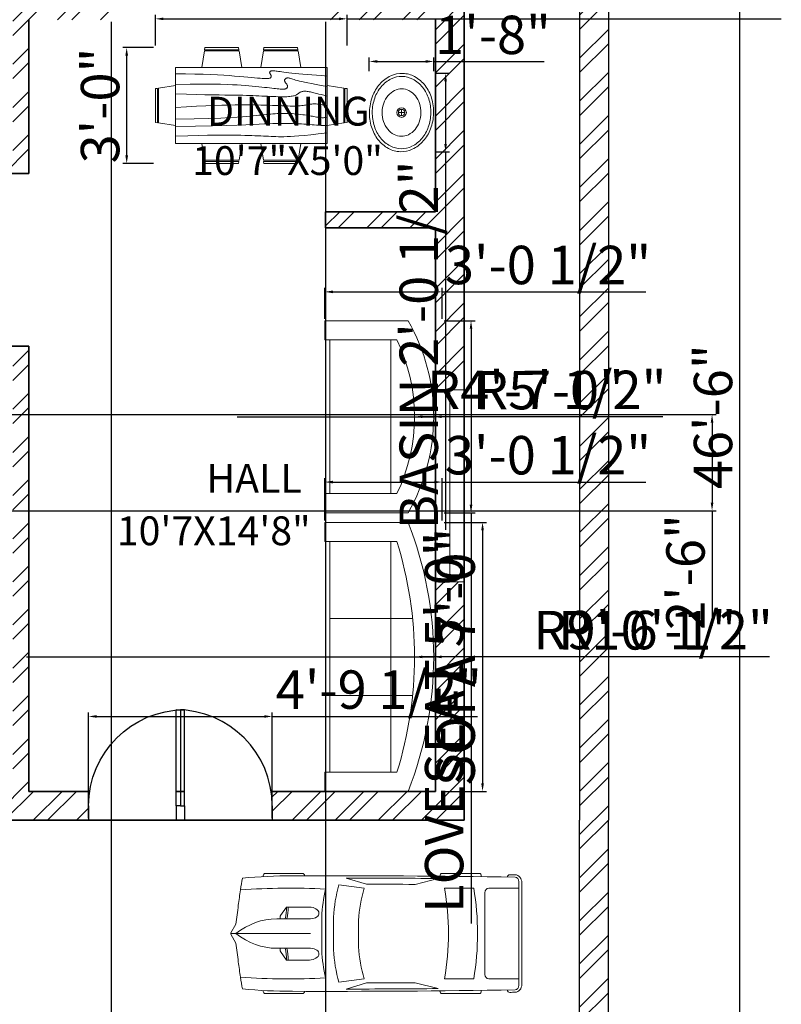
# Model space of a CAD drawing. Units: inches. Extents: x 2588 to 3237, y 2402 to 3178.
# Tile 3 of 4: x 2878 to 3115, y 2568 to 2876. Entities that reach past the tile are written whole.
import ezdxf

# ---------------------------------------------------------------- set-up
doc = ezdxf.new("R2010")
doc.units = ezdxf.units.IN
for name, color, linetype, lineweight in [('A-ANNO-DIMS', 2, 'Continuous', 18), ('A-AREA-IDEN', 7, 'Continuous', 25), ('A-DOOR', 3, 'Continuous', 25), ('A-FLOR-FIXT', 9, 'Continuous', 18), ('A-FURN', 8, 'Continuous', 18), ('A-GLAZ', 4, 'Continuous', 18), ('A-WALL-PATT', 252, 'Continuous', 13), ('C-PRKG-VEHI', 8, 'Continuous', 18), ('L-WALL', 7, 'Continuous', 30), ('L-WALL-PATT', 252, 'Continuous', 13), ('wall', 210, 'Continuous', 35)]:
    doc.layers.add(name, color=color, linetype=linetype, lineweight=lineweight)
doc.styles.get("Standard").update_dxf_attribs({"font": 'arial.ttf'})
doc.dimstyles.new('ISO-25', dxfattribs={"dimtxt": 12, "dimasz": 2.5, "dimexe": 1.25, "dimexo": 0.625, "dimtad": 1, "dimdec": 1, "dimlunit": 4, "dimtxsty": 'Standard', "dimcen": 2.5, "dimadec": 0, "dimazin": 0, "dimtfac": 1, "dimtdec": 1, "dimtmove": 0, "dimatfit": 3, "dimfxl": 1, "dimarcsym": 0})

# ---------------------------------------------------------------- blocks, each defined once
blk = doc.blocks.new('Dining Set - 36 x 72 in.')
for p, q in [((-22.2343, 26.00059), (-23.4847, 17.99762)), ((-22.2304, 26), (-5.7608, 26)), ((-22, 27.5), (-22.1562, 26.50042)), ((-5.8416, 26.5), (-22.1534, 26.5)), ((-22, 27.5), (-6, 27.5)), ((-5.8437, 26.49966), (-6, 27.5)), ((-4.5152, 17.99762), (-5.7655, 25.99926)), ((5.7657, 26.00059), (4.5153, 17.99762)), ((5.7696, 26), (22.2392, 26)), ((6, 27.5), (5.8438, 26.50042)), ((22.1584, 26.5), (5.8466, 26.5)), ((6, 27.5), (22, 27.5)), ((22.1563, 26.49966), (22, 27.5)), ((23.4848, 17.99762), (22.2345, 25.99926)), ((36, 18), (-36, 18)), ((-36, 18), (-36, -18)), ((36, -18), (36, 18)), ((-44.0006, 8.23428), (-35.9976, 9.48474)), ((44.0006, 8.23428), (35.9976, 9.48474)), ((-45.5, 8), (-44.5004, 8.15617)), ((-45.5, 8), (-45.5, -8)), ((-44.5, -8.15843), (-44.5, 8.15338)), ((-44, 8.23041), (-44, -8.23915)), ((44, 8.23041), (44, -8.23915)), ((44.5, -8.15843), (44.5, 8.15338)), ((45.5, 8), (44.5005, 8.15617)), ((45.5, 8), (45.5, -8)), ((-44.4997, -8.15631), (-45.5, -8)), ((-35.9976, -9.48476), (-43.9993, -8.2345)), ((35.9976, -9.48476), (43.9993, -8.2345)), ((44.4997, -8.15631), (45.5, -8)), ((-36, -18), (36, -18)), ((-22.2343, -26.0006), (-23.4847, -17.99762)), ((-4.5152, -17.99762), (-5.7655, -25.99928)), ((5.7657, -26.0006), (4.5153, -17.99762)), ((23.4848, -17.99762), (22.2345, -25.99928)), ((-22.2304, -26), (-5.7608, -26)), ((-22, -27.5), (-22.1562, -26.50044)), ((-5.8416, -26.5), (-22.1534, -26.5)), ((-22, -27.5), (-6, -27.5)), ((-5.8437, -26.49967), (-6, -27.5)), ((5.7696, -26), (22.2392, -26)), ((6, -27.5), (5.8438, -26.50044)), ((22.1584, -26.5), (5.8466, -26.5)), ((6, -27.5), (22, -27.5)), ((22.1563, -26.49967), (22, -27.5))]:
    blk.add_line(p, q)
for points in [[(-36, 15), (-31.1772, 14.97754), (-26.8079, 14.91406), (-22.8538, 14.81543), (-19.276, 14.6875), (-16.0362, 14.53613), (-13.0957, 14.36718), (-10.4159, 14.18652), (-7.9583, 14), (-5.6904, 13.81315), (-3.6035, 13.63021), (-1.6954, 13.45508), (0.0365, 13.29166), (1.5945, 13.14388), (2.9811, 13.01562), (4.1988, 12.9108), (5.25, 12.83333), (6.1393, 12.78613), (6.8802, 12.76823), (7.4883, 12.77767), (7.9792, 12.8125), (8.3685, 12.87077), (8.6719, 12.95052), (8.9049, 13.0498), (9.0833, 13.16666), (9.2205, 13.29899), (9.3216, 13.44401), (9.3895, 13.59879), (9.4271, 13.76041), (9.4373, 13.92594), (9.4232, 14.09245), (9.3875, 14.257), (9.3333, 14.41666), (9.2638, 14.56917), (9.1836, 14.71484), (9.0975, 14.85465), (9.0104, 14.98958), (8.9272, 15.1206), (8.8529, 15.2487), (8.7922, 15.37483), (8.75, 15.5), (8.7305, 15.62467), (8.7344, 15.74739), (8.7617, 15.86621), (8.8125, 15.97916), (8.8867, 16.08431), (8.9844, 16.17968), (9.1055, 16.26334), (9.25, 16.33333), (9.4189, 16.38802), (9.6172, 16.42708), (9.8506, 16.45052), (10.125, 16.45833), (10.4463, 16.45052), (10.8203, 16.42708), (11.2529, 16.38802), (11.75, 16.33333), (12.3184, 16.26318), (12.9694, 16.17838), (13.7151, 16.07991), (14.5677, 15.96875), (15.5395, 15.84586), (16.6426, 15.71224), (17.8893, 15.56884), (19.2917, 15.41666), (20.859, 15.25667), (22.5879, 15.08984), (24.4721, 14.91715), (26.5052, 14.73958), (28.6809, 14.5581), (30.9929, 14.3737), (33.4347, 14.18733), (36, 14)], [(-36, 10), (-28.9766, 10.14274), (-23.1725, 10.20442), (-18.4241, 10.19775), (-14.5677, 10.13541), (-11.4399, 10.03011), (-8.877, 9.89453), (-6.7154, 9.74137), (-4.7917, 9.58333), (-2.9698, 9.43082), (-1.2246, 9.28515), (0.4415, 9.14534), (2.026, 9.01041), (3.5266, 8.87939), (4.9408, 8.7513), (6.266, 8.62516), (7.5, 8.5), (8.6411, 8.37549), (9.6914, 8.2539), (10.6538, 8.13818), (11.5312, 8.03125), (12.3267, 7.93603), (13.043, 7.85547), (13.6831, 7.79248), (14.25, 7.75), (14.7471, 7.7303), (15.1797, 7.73307), (15.5537, 7.75732), (15.875, 7.80208), (16.1494, 7.86637), (16.3828, 7.94922), (16.5811, 8.04964), (16.75, 8.16666), (16.8944, 8.29915), (17.0143, 8.44531), (17.1089, 8.60319), (17.1771, 8.77083), (17.218, 8.94629), (17.2305, 9.1276), (17.2137, 9.31282), (17.1667, 9.5), (17.0895, 9.6875), (16.987, 9.875), (16.8649, 10.0625), (16.7292, 10.25), (16.5856, 10.4375), (16.4401, 10.625), (16.2985, 10.8125), (16.1667, 11), (16.05, 11.18733), (15.9518, 11.3737), (15.8752, 11.5581), (15.8229, 11.73958), (15.798, 11.91715), (15.8034, 12.08984), (15.842, 12.25667), (15.9167, 12.41666), (16.0295, 12.56836), (16.1784, 12.70833), (16.3605, 12.83268), (16.5729, 12.9375), (16.8127, 13.01888), (17.0768, 13.07291), (17.3625, 13.0957), (17.6667, 13.08333), (17.9894, 13.03312), (18.3418, 12.94726), (18.7382, 12.82918), (19.1927, 12.68229), (19.7195, 12.51001), (20.3327, 12.31575), (21.0465, 12.10294), (21.875, 11.875), (22.8357, 11.63354), (23.959, 11.37304), (25.2786, 11.08618), (26.8282, 10.76562), (28.6414, 10.40405), (30.752, 9.99414), (33.1936, 9.52856), (36, 9)], [(-36, 5.5), (-30.7157, 5.3348), (-26.069, 5.20963), (-21.9946, 5.11767), (-18.4271, 5.05208), (-15.3009, 5.00602), (-12.5508, 4.97265), (-10.1112, 4.94515), (-7.9167, 4.91666), (-5.909, 4.88167), (-4.0586, 4.83984), (-2.3429, 4.79215), (-0.7396, 4.73958), (0.7739, 4.6831), (2.22, 4.6237), (3.6213, 4.56233), (5, 4.5), (6.373, 4.43782), (7.7344, 4.3776), (9.0723, 4.32129), (10.375, 4.27083), (11.6309, 4.22819), (12.8281, 4.19531), (13.9551, 4.17415), (15, 4.16666), (15.954, 4.17448), (16.819, 4.19791), (17.6001, 4.23698), (18.3021, 4.29166), (18.9299, 4.36198), (19.4883, 4.44791), (19.9823, 4.54948), (20.4167, 4.66666), (20.7969, 4.79899), (21.1302, 4.94401), (21.4245, 5.09879), (21.6875, 5.26041), (21.9271, 5.42594), (22.1511, 5.59245), (22.3672, 5.757), (22.5834, 5.91666), (22.8065, 6.06868), (23.0404, 6.21093), (23.2879, 6.34147), (23.5521, 6.45833), (23.8358, 6.55957), (24.142, 6.64323), (24.4735, 6.70735), (24.8334, 6.75), (25.2235, 6.76969), (25.642, 6.76692), (26.0858, 6.74267), (26.5521, 6.69791), (27.0379, 6.63362), (27.5404, 6.55078), (28.0565, 6.45036), (28.5834, 6.33333), (29.1242, 6.19987), (29.7071, 6.04687), (30.3661, 5.87044), (31.1354, 5.66666), (32.0493, 5.43164), (33.142, 5.16146), (34.4475, 4.85221), (36, 4.5)], [(-36, -1), (-30.7915, -0.6591), (-26.0195, -0.38216), (-21.6519, -0.16284), (-17.6563, 0.00521), (-14.0005, 0.12833), (-10.6523, 0.21289), (-7.5796, 0.26522), (-4.75, 0.29166), (-2.134, 0.29793), (0.2878, 0.28711), (2.5317, 0.26163), (4.6146, 0.22396), (6.5529, 0.17651), (8.3633, 0.12174), (10.0623, 0.06209), (11.6667, 0), (13.1899, -0.06201), (14.6341, -0.1211), (15.9982, -0.17432), (17.2813, -0.21875), (18.4823, -0.25147), (19.6003, -0.26953), (20.6343, -0.27002), (21.5834, -0.25), (22.4481, -0.20768), (23.2357, -0.14584), (23.9549, -0.06836), (24.6146, 0.02083), (25.2235, 0.11784), (25.7904, 0.21875), (26.3241, 0.31966), (26.8334, 0.41666), (27.3265, 0.50618), (27.8099, 0.58593), (28.2894, 0.65397), (28.7709, 0.70833), (29.2601, 0.74707), (29.763, 0.76823), (30.2855, 0.76985), (30.8334, 0.75), (31.4088, 0.70784), (31.9994, 0.64713), (32.589, 0.57275), (33.1615, 0.48958), (33.7008, 0.4025), (34.1908, 0.3164), (34.6153, 0.23616), (34.9584, 0.16666), (35.2099, 0.11165), (35.3848, 0.07031), (35.504, 0.04069), (35.5886, 0.02083), (35.6594, 0.00879), (35.7377, 0.0026), (35.8442, 0.00032), (36, 0)], [(-36, -6.5), (-27.1843, -6.31267), (-20.084, -6.1263), (-14.469, -5.9419), (-10.1094, -5.76042), (-6.7752, -5.58285), (-4.2363, -5.41016), (-2.2629, -5.24333), (-0.625, -5.08334), (0.8708, -4.93099), (2.2715, -4.78646), (3.5872, -4.64974), (4.8281, -4.52084), (6.0046, -4.39974), (7.127, -4.28646), (8.2053, -4.18099), (9.25, -4.08334), (10.2705, -3.99382), (11.2734, -3.91407), (12.2647, -3.84603), (13.25, -3.79167), (14.2354, -3.75293), (15.2266, -3.73177), (16.2295, -3.73015), (17.25, -3.75), (18.2912, -3.79248), (19.3451, -3.85547), (20.4009, -3.93604), (21.4479, -4.03125), (22.4754, -4.13819), (23.4727, -4.25391), (24.4289, -4.37549), (25.3334, -4.5), (26.1785, -4.62492), (26.9694, -4.74935), (27.7145, -4.87281), (28.4219, -4.99479), (29.1, -5.11483), (29.7572, -5.23242), (30.4016, -5.34709), (31.0417, -5.45834), (31.6837, -5.56437), (32.3262, -5.65821), (32.9658, -5.73153), (33.599, -5.77604), (34.2224, -5.78345), (34.8327, -5.74545), (35.4264, -5.65373), (36, -5.5)], [(-36, -10), (-26.4022, -9.81299), (-18.4675, -9.62891), (-11.9839, -9.45069), (-6.7396, -9.28125), (-2.5226, -9.12354), (0.8789, -8.98047), (3.6769, -8.85498), (6.0833, -8.75), (8.2767, -8.66765), (10.3021, -8.60677), (12.1712, -8.56543), (13.8958, -8.54167), (15.4876, -8.53353), (16.9583, -8.53907), (18.3197, -8.55632), (19.5834, -8.58334), (20.7616, -8.61841), (21.8685, -8.66081), (22.9188, -8.71004), (23.9271, -8.76563), (24.9081, -8.82707), (25.8763, -8.89388), (26.8465, -8.96558), (27.8334, -9.04167), (28.8474, -9.12118), (29.8828, -9.20117), (30.93, -9.27824), (31.9792, -9.34896), (33.0205, -9.40991), (34.0443, -9.45768), (35.0407, -9.48885), (36, -9.5)], [(-36, -14.5), (-30.0881, -14.33513), (-25.0332, -14.21224), (-20.7312, -14.12647), (-17.0781, -14.07292), (-13.97, -14.04671), (-11.3027, -14.04297), (-8.9724, -14.05681), (-6.875, -14.08334), (-4.9224, -14.11833), (-3.0905, -14.16016), (-1.3709, -14.20785), (0.2448, -14.26042), (1.7647, -14.3169), (3.1973, -14.3763), (4.5507, -14.43767), (5.8333, -14.5), (7.0554, -14.5621), (8.235, -14.62175), (9.3922, -14.67652), (10.5469, -14.72396), (11.7192, -14.76164), (12.929, -14.78711), (14.1965, -14.79794), (15.5417, -14.79167), (16.9933, -14.76424), (18.6152, -14.70508), (20.4804, -14.60197), (22.6615, -14.44271), (25.2312, -14.21509), (28.2624, -13.9069), (31.8277, -13.50594), (36, -13)]]:
    blk.add_lwpolyline(points)
blk = doc.blocks.new('Sink - Oval top')
for p, q in [((-1, 0), (1, 0)), ((0, 1), (0, -1))]:
    blk.add_line(p, q)
for points in [[(-12.23, 0.39, 0.117634), (-11.46, -3.36, 0.104469), (-8.88, -6.8, 0.090016), (-5.08, -9.07, 0.08192), (-0.32, -10.02, 0.08192), (4.49, -9.38, 0.090016), (8.42, -7.36, 0.104469), (11.22, -4.09, 0.117634), (12.23, -0.39, 0.117634), (11.46, 3.36, 0.104469), (8.88, 6.8, 0.090016), (5.08, 9.07, 0.08192), (0.32, 10.02, 0.08192), (-4.49, 9.38, 0.090016), (-8.42, 7.36, 0.104469), (-11.22, 4.09, 0.117634)], [(-11.29, 0.16, 0.118622), (-10.52, -3.25, 0.104678), (-8.07, -6.36, 0.089562), (-4.54, -8.37, 0.081185), (-0.13, -9.15, 0.081185), (4.3, -8.49, 0.089562), (7.89, -6.58, 0.104678), (10.42, -3.55, 0.118622), (11.29, -0.16, 0.118622), (10.52, 3.25, 0.104678), (8.07, 6.36, 0.089562), (4.54, 8.37, 0.081185), (0.13, 9.15, 0.081185), (-4.3, 8.49, 0.089562), (-7.89, 6.58, 0.104678), (-10.42, 3.55, 0.118622)], [(-7.42, 0.08, 0.118283), (-6.91, -2.17, 0.104607), (-5.29, -4.21, 0.089718), (-2.97, -5.53, 0.081436), (-0.07, -6.04, 0.081436), (2.84, -5.59, 0.089718), (5.2, -4.33, 0.104607), (6.86, -2.32, 0.118283), (7.42, -0.08, 0.118283), (6.91, 2.17, 0.104607), (5.29, 4.21, 0.089718), (2.97, 5.53, 0.081436), (0.07, 6.04, 0.081436), (-2.84, 5.59, 0.089718), (-5.2, 4.33, 0.104607), (-6.86, 2.32, 0.118283)]]:
    blk.add_lwpolyline(points, format="xyb", close=True)
for radius in [1.5, 1]:
    blk.add_circle((0, 0), radius)
blk = doc.blocks.new('*U14')
for p, q in [((0, 0), (0, -6)), ((40, 0), (40, -6))]:
    blk.add_line(p, q)
blk.add_lwpolyline([(0, 0), (0, 40), (1.75, 40), (1.75, 0)], close=True)
blk.add_arc((0, 0), 40, 0, 90)
blk = doc.blocks.new('Sofa - Roundback 7 ft.')
for p, q in [((-12.00002, -32.4421), (-12.00003, -6.5971)), ((11.99997, -32.4421), (11.99998, -6.5971)), ((-36.000027, -34), (-36.000027, -11.4696)), ((35.99998, -34), (35.99998, -11.4696)), ((-35.999844, -13.3819), (35.9998, -13.3819)), ((-36.000027, -32.4421), (35.99998, -32.4421))]:
    blk.add_line(p, q)
for points in [[(-36.000027, -34), (-42.000027, -34), (-42.000027, -8)], [(41.99998, -8), (41.99998, -34), (35.99998, -34)]]:
    blk.add_lwpolyline(points)
for centre, radius, start, end in [((0, -114.25), 114.25, 68.43141, 111.5686), ((-0.00001, -127.1968), 121.1968, 72.72033, 107.2797)]:
    blk.add_arc(centre, radius, start, end)
blk = doc.blocks.new('Sofa - Roundback Loveseat 5 ft.')
for p, q in [((0, -32.44198), (0, -5.99998)), ((-24, -33.99998), (-24, -11.46958)), ((24.00004, -33.99998), (24.00004, -11.46958)), ((-23.9998, -13.38178), (23.99986, -13.38178)), ((-24, -32.44198), (24.00004, -32.44198))]:
    blk.add_line(p, q)
for points in [[(-24, -33.99998), (-30, -33.99998), (-30, -7.99998)], [(30.00004, -7.99998), (30.00004, -33.99998), (24.00004, -33.99998)]]:
    blk.add_lwpolyline(points)
for centre, radius, start, end in [((0, -60.24998), 60.24998, 60.13715, 119.8628), ((0, -61.38438), 55.38444, 64.32083, 115.6792)]:
    blk.add_arc(centre, radius, start, end)
blk = doc.blocks.new('*U21')
for p, q in [((46.55, 38.89), (22.35, 38.89)), ((136.7, 38.89), (160.9, 38.89)), ((21.1, 37.41), (21.1, 36.83)), ((47.8, 37.39), (47.8, 37.41)), ((87.99, 31.87), (74.76, 35.92)), ((134.31, 35.6), (119.29, 31.78)), ((135.45, 37.07), (135.45, 37.41)), ((162.15, 37.41), (162.15, 36.77)), ((186.47, -33.5), (186.47, 33.5)), ((188.4, -32.76), (188.4, 32.76)), ((70.03, 31.54), (86.41, 29.35)), ((138.42, 29.35), (157.25, 29.35)), ((164.52, 26.39), (164.52, -26.39)), ((186.47, 29.35), (167.01, 29.35)), ((32.27, 11.63), (36.13, 17.17)), ((36.13, 17.17), (50.94, 17.17)), ((29.77, 9.51), (51.68, 9.51)), ((32.12, 9.51), (32.12, 11.15)), ((58.92, -10.77), (58.92, 10.77)), ((66.55, -10.53), (66.55, 10.53)), ((82.74, 8.5), (82.74, -8.5)), ((186.47, -10.53), (186.47, 10.53)), ((3.27, 6.13), (0.1, 0.41)), ((0, 0), (51.68, 0)), ((0.1, -0.41), (3.27, -6.13)), ((29.77, -9.51), (51.68, -9.51)), ((32.12, -9.51), (32.12, -11.15)), ((32.27, -11.63), (36.13, -17.17)), ((36.13, -17.17), (50.94, -17.17)), ((86.41, -29.35), (70.03, -31.54)), ((134.31, -35.6), (119.29, -31.78)), ((157.25, -29.35), (138.42, -29.35)), ((167.01, -29.35), (186.47, -29.35)), ((21.1, -37.41), (21.1, -36.83)), ((47.8, -37.39), (47.8, -37.41)), ((87.99, -31.87), (74.76, -35.92)), ((135.45, -37.07), (135.45, -37.41)), ((162.15, -37.41), (162.15, -36.77)), ((46.55, -38.89), (22.35, -38.89)), ((136.7, -38.89), (160.9, -38.89))]:
    blk.add_line(p, q)
for centre, major_axis, ratio, start_param, end_param in [((22.35, 37.41), (0, -1.48), 0.842304, 3.141593, 4.712389), ((46.55, 37.41), (0, 1.48), 0.842304, -1.570796, 0), ((136.7, 37.41), (0, -1.48), 0.842304, 3.141593, 4.712389), ((160.9, 37.41), (0, 1.48), 0.842304, -1.570796, 0), ((266.03, -27.52), (0, 313.31), 0.842304, 1.367076, 1.39176), ((41.19, -490.86), (0, 528.23), 0.842304, 0.00281, 0.075598), ((64.48, -10555.62), (0, 10593.03), 0.842304, -0.013397, 0.002797), ((64.48, -10555.62), (0, -10591.55), 0.842304, 3.133765, 3.140441), ((95.79, -3666.35), (0, -3698.24), 0.842304, 3.134049, 3.144098), ((180.63, 35.84), (0, 2.22), 0.842304, -0.013017, 1.249894), ((64.48, -10556.36), (0, 10595.31), 0.842304, -0.013397, -0.013017), ((183.98, 33.5), (0, -2.96), 0.842304, 1.570796, 3.128196), ((183.98, 32.76), (0, -5.25), 0.842304, 1.570796, 3.128196), ((259.18, -27.52), (0, -305.3), 0.842304, 4.528606, 4.561838), ((37.47, -593.96), (0, -623.33), 0.842304, 3.096046, 3.200911), ((134.4, 5.39), (0, -89.78), 0.842304, 4.449482, 4.652344), ((135.29, 5.39), (0, 81.77), 0.842304, 1.245306, 1.50788), ((149.6, 2.8), (0, -79.58), 0.842304, 4.372215, 4.640744), ((17.08, 0), (0, 147.02), 0.842304, 4.511394, 4.913384), ((35.91, 0), (0, 147.02), 0.842304, 4.511394, 4.913384), ((167.01, 26.39), (0, 2.96), 0.842304, 0, 1.570796), ((-204.49, 52.4), (0, -250.96), 0.842304, 1.385369, 1.434372), ((13.04, 17.01), (0, 27.42), 0.842304, 4.435146, 4.718221), ((14.2, 17.01), (0, 27.42), 0.842304, 4.435146, 4.718221), ((50.79, 13.34), (6.34, -0.36), 0.603834, -1.395552, 1.581315), ((29.77, -46.66), (0, 56.17), 0.842304, 0, 0.590319), ((32.75, 11.15), (0, 0.74), 0.842304, 0.879714, 1.570796), ((0.62, 0), (0, -0.74), 0.842304, 4.131459, 5.293319), ((-204.49, -52.4), (0, 250.96), 0.842304, -1.434372, -1.385369), ((29.77, 46.66), (0, 56.17), 0.842304, 2.551274, 3.141593), ((32.75, -11.15), (0, -0.74), 0.842304, 4.712389, 5.403472), ((13.04, -17.01), (0, -27.42), 0.842304, 1.564964, 1.848039), ((14.2, -17.01), (0, -27.42), 0.842304, 1.564964, 1.848039), ((134.4, -5.39), (0, -89.78), 0.842304, -1.510751, -1.307889), ((135.29, -5.39), (0, -81.77), 0.842304, -1.50788, -1.245306), ((149.6, -2.8), (0, -79.58), 0.842304, -1.499151, -1.230623), ((259.18, 27.52), (0, 305.3), 0.842304, 1.721348, 1.754579), ((266.03, 27.52), (0, 313.31), 0.842304, 1.749832, 1.774517), ((37.47, 593.96), (0, -623.33), 0.842304, -0.059319, 0.045547), ((95.79, 3666.35), (0, -3698.24), 0.842304, -0.002505, 0.007544), ((167.01, -26.39), (0, -2.96), 0.842304, 4.712389, 6.283185), ((41.19, 490.86), (0, -528.23), 0.842304, -0.075598, -0.00281), ((22.35, -37.41), (0, 1.48), 0.842304, 1.570796, 3.141593), ((64.48, 10555.62), (0, 10593.03), 0.842304, 3.138796, 3.15499), ((46.55, -37.41), (0, -1.48), 0.842304, 0, 1.570796), ((64.48, 10555.62), (0, -10591.55), 0.842304, 0.001152, 0.007828), ((136.7, -37.41), (0, -1.48), 0.842304, -1.570796, 0), ((160.9, -37.41), (0, 1.48), 0.842304, 3.141593, 4.712389), ((180.63, -35.84), (0, -2.22), 0.842304, -1.249894, 0.013017), ((64.48, 10556.36), (0, 10595.31), 0.842304, 3.15461, 3.15499), ((183.98, -33.5), (0, 2.96), 0.842304, 3.15499, 4.712389), ((183.98, -32.76), (0, -5.25), 0.842304, 0.013397, 1.570796)]:
    blk.add_ellipse(centre, major_axis=major_axis, ratio=ratio, start_param=start_param, end_param=end_param)
at = {"extrusion": (0, 0, -1)}
blk.add_ellipse((50.79, -13.34), major_axis=(6.34, 0.36), ratio=0.603834, start_param=-1.395552, end_param=1.581315, dxfattribs=at)
blk = doc.blocks.new('*D23')
at = {"layer": 'A-ANNO-DIMS', "color": 0, "lineweight": -2, "transparency": 16777216}
for p, q in [((3062.02, 3030.83), (3103.65, 3030.83)), ((3102.4, 3028.33), (3102.4, 2475.33)), ((3062.02, 2472.83), (3103.65, 2472.83))]:
    blk.add_line(p, q, dxfattribs=at)
at = {"layer": 'A-ANNO-DIMS', "color": 0, "transparency": 16777216}
for points in [[(3101.99, 3028.33), (3102.82, 3028.33), (3102.4, 3030.83)], [(3101.99, 2475.33), (3102.82, 2475.33), (3102.4, 2472.83)]]:
    blk.add_solid(points, dxfattribs=at)
at = {"layer": 'Defpoints', "color": 0, "transparency": 16777216}
for p in [(3061.4, 3030.83), (3061.4, 2472.83), (3102.4, 2472.83)]:
    blk.add_point(p, dxfattribs=at)
at = {"layer": 'A-ANNO-DIMS', "color": 0, "transparency": 16777216, "insert": (3095.65, 2751.83), "char_height": 12, "attachment_point": 5, "rotation": 90}
blk.add_mtext('46\'-6"', dxfattribs=at)
blk = doc.blocks.new('WIN-60IN')
blk.add_line((4.5, 60), (4.5, 0))
blk.add_lwpolyline([(9, 60), (9, 0), (0, 0), (0, 60)], close=True)
blk = doc.blocks.new('*D29')
at = {"layer": 'A-ANNO-DIMS', "color": 0, "lineweight": -2, "transparency": 16777216}
for p, q in [((2761.13, 2894.89), (2761.13, 2882.27)), ((2821.13, 2894.89), (2821.13, 2882.27)), ((2763.63, 2883.52), (2818.63, 2883.52)), ((2821.13, 2883.52), (2898.03, 2883.52))]:
    blk.add_line(p, q, dxfattribs=at)
at = {"layer": 'A-ANNO-DIMS', "color": 0, "transparency": 16777216}
for points in [[(2763.63, 2883.93), (2763.63, 2883.1), (2761.13, 2883.52)], [(2818.63, 2883.93), (2818.63, 2883.1), (2821.13, 2883.52)]]:
    blk.add_solid(points, dxfattribs=at)
at = {"layer": 'Defpoints', "color": 0, "transparency": 16777216}
for p in [(2761.13, 2895.52), (2821.13, 2895.52), (2821.13, 2883.52)]:
    blk.add_point(p, dxfattribs=at)
at = {"layer": 'A-ANNO-DIMS', "color": 0, "transparency": 16777216, "insert": (2860.83, 2890.27), "char_height": 12, "attachment_point": 5}
blk.add_mtext('5\'-0" TYP.', dxfattribs=at)
blk = doc.blocks.new('*D36')
at = {"layer": 'A-ANNO-DIMS', "color": 0, "lineweight": -2, "transparency": 16777216}
for p, q in [((2919.92, 2867.74), (2919.92, 2877.35)), ((2922.42, 2876.1), (2977.29, 2876.1)), ((2979.79, 2867.74), (2979.79, 2877.35)), ((2979.79, 2876.1), (3115.43, 2876.1))]:
    blk.add_line(p, q, dxfattribs=at)
at = {"layer": 'A-ANNO-DIMS', "color": 0, "transparency": 16777216}
for points in [[(2922.42, 2876.51), (2922.42, 2875.68), (2919.92, 2876.1)], [(2977.29, 2876.51), (2977.29, 2875.68), (2979.79, 2876.1)]]:
    blk.add_solid(points, dxfattribs=at)
at = {"layer": 'Defpoints', "color": 0, "transparency": 16777216}
for p in [(2979.79, 2876.1), (2919.92, 2867.12), (2979.79, 2867.12)]:
    blk.add_point(p, dxfattribs=at)
at = {"layer": 'A-ANNO-DIMS', "color": 0, "transparency": 16777216, "insert": (3048.86, 2882.93), "char_height": 12, "attachment_point": 5}
blk.add_mtext('DINING SET 5\'-0"', dxfattribs=at)
blk = doc.blocks.new('*D37')
at = {"layer": 'A-ANNO-DIMS', "color": 0, "lineweight": -2, "transparency": 16777216}
for p, q in [((2919.3, 2867.12), (2909.69, 2867.12)), ((2910.94, 2833.44), (2910.94, 2864.62)), ((2919.3, 2830.94), (2909.69, 2830.94))]:
    blk.add_line(p, q, dxfattribs=at)
at = {"layer": 'A-ANNO-DIMS', "color": 0, "transparency": 16777216}
for points in [[(2910.53, 2864.62), (2911.36, 2864.62), (2910.94, 2867.12)], [(2910.53, 2833.44), (2911.36, 2833.44), (2910.94, 2830.94)]]:
    blk.add_solid(points, dxfattribs=at)
at = {"layer": 'Defpoints', "color": 0, "transparency": 16777216}
for p in [(2910.94, 2867.12), (2919.92, 2867.12), (2919.92, 2830.94)]:
    blk.add_point(p, dxfattribs=at)
at = {"layer": 'A-ANNO-DIMS', "color": 0, "transparency": 16777216, "insert": (2904.19, 2849.03), "char_height": 12, "attachment_point": 5, "rotation": 90}
blk.add_mtext('3\'-0"', dxfattribs=at)
blk = doc.blocks.new('*D38')
at = {"layer": 'A-ANNO-DIMS', "color": 0, "lineweight": -2, "transparency": 16777216}
for p, q in [((3007.49, 2859.11), (3011.8, 2859.11)), ((3010.55, 2856.61), (3010.55, 2837.06)), ((3007.49, 2834.56), (3011.8, 2834.56)), ((3010.55, 2834.56), (3010.55, 2716.51))]:
    blk.add_line(p, q, dxfattribs=at)
at = {"layer": 'A-ANNO-DIMS', "color": 0, "transparency": 16777216}
for points in [[(3010.14, 2856.61), (3010.97, 2856.61), (3010.55, 2859.11)], [(3010.14, 2837.06), (3010.97, 2837.06), (3010.55, 2834.56)]]:
    blk.add_solid(points, dxfattribs=at)
at = {"layer": 'Defpoints', "color": 0, "transparency": 16777216}
for p in [(3006.87, 2859.11), (3006.87, 2834.56), (3010.55, 2834.56)]:
    blk.add_point(p, dxfattribs=at)
at = {"layer": 'A-ANNO-DIMS', "color": 0, "transparency": 16777216, "insert": (3003.72, 2774.28), "char_height": 12, "attachment_point": 5, "rotation": 90}
blk.add_mtext('BASIN 2\'-0 1/2"', dxfattribs=at)
blk = doc.blocks.new('*D39')
at = {"layer": 'A-ANNO-DIMS', "color": 0, "lineweight": -2, "transparency": 16777216}
for p, q in [((2986.73, 2859.73), (2986.73, 2864.04)), ((2989.23, 2862.79), (3004.37, 2862.79)), ((3006.87, 2859.73), (3006.87, 2864.04)), ((3006.87, 2862.79), (3041.39, 2862.79))]:
    blk.add_line(p, q, dxfattribs=at)
at = {"layer": 'A-ANNO-DIMS', "color": 0, "transparency": 16777216}
for points in [[(2989.23, 2863.21), (2989.23, 2862.37), (2986.73, 2862.79)], [(3004.37, 2863.21), (3004.37, 2862.37), (3006.87, 2862.79)]]:
    blk.add_solid(points, dxfattribs=at)
at = {"layer": 'Defpoints', "color": 0, "transparency": 16777216}
for p in [(3006.87, 2862.79), (2986.73, 2859.11), (3006.87, 2859.11)]:
    blk.add_point(p, dxfattribs=at)
at = {"layer": 'A-ANNO-DIMS', "color": 0, "transparency": 16777216, "insert": (3025.38, 2869.54), "char_height": 12, "attachment_point": 5}
blk.add_mtext('1\'-8"', dxfattribs=at)
blk = doc.blocks.new('*D42')
at = {"layer": 'A-ANNO-DIMS', "color": 0, "lineweight": -2, "transparency": 16777216}
for p, q in [((3010.13, 2718.83), (3023.36, 2718.83)), ((3022.11, 2716.33), (3022.11, 2637.33)), ((3010.13, 2634.83), (3023.36, 2634.83))]:
    blk.add_line(p, q, dxfattribs=at)
at = {"layer": 'A-ANNO-DIMS', "color": 0, "transparency": 16777216}
for points in [[(3021.69, 2716.33), (3022.52, 2716.33), (3022.11, 2718.83)], [(3021.69, 2637.33), (3022.52, 2637.33), (3022.11, 2634.83)]]:
    blk.add_solid(points, dxfattribs=at)
at = {"layer": 'Defpoints', "color": 0, "transparency": 16777216}
for p in [(3009.51, 2718.83), (3009.51, 2634.83), (3022.11, 2634.83)]:
    blk.add_point(p, dxfattribs=at)
at = {"layer": 'A-ANNO-DIMS', "color": 0, "transparency": 16777216, "insert": (3015.27, 2676.83), "char_height": 12, "attachment_point": 5, "rotation": 90}
blk.add_mtext('SOFA 7\'-0"', dxfattribs=at)
blk = doc.blocks.new('*D43')
at = {"layer": 'A-ANNO-DIMS', "color": 0, "lineweight": -2, "transparency": 16777216}
for p, q in [((2972.84, 2719.46), (2972.84, 2732.68)), ((2975.34, 2731.43), (3007.01, 2731.43)), ((3009.51, 2719.46), (3009.51, 2732.68)), ((3009.51, 2731.43), (3073.11, 2731.43))]:
    blk.add_line(p, q, dxfattribs=at)
at = {"layer": 'A-ANNO-DIMS', "color": 0, "transparency": 16777216}
for points in [[(2975.34, 2731.85), (2975.34, 2731.02), (2972.84, 2731.43)], [(3007.01, 2731.85), (3007.01, 2731.02), (3009.51, 2731.43)]]:
    blk.add_solid(points, dxfattribs=at)
at = {"layer": 'Defpoints', "color": 0, "transparency": 16777216}
for p in [(3009.51, 2731.43), (2972.84, 2718.83), (3009.51, 2718.83)]:
    blk.add_point(p, dxfattribs=at)
at = {"layer": 'A-ANNO-DIMS', "color": 0, "transparency": 16777216, "insert": (3042.56, 2738.27), "char_height": 12, "attachment_point": 5}
blk.add_mtext('3\'-0 1/2"', dxfattribs=at)
blk = doc.blocks.new('*D44')
at = {"layer": 'A-ANNO-DIMS', "color": 0, "lineweight": -2, "transparency": 16777216}
for p, q in [((3010.13, 2781.83), (3019.76, 2781.83)), ((3018.51, 2779.33), (3018.51, 2724.33)), ((3010.13, 2721.83), (3019.76, 2721.83)), ((3018.51, 2721.83), (3018.51, 2593.55))]:
    blk.add_line(p, q, dxfattribs=at)
at = {"layer": 'A-ANNO-DIMS', "color": 0, "transparency": 16777216}
for points in [[(3018.09, 2779.33), (3018.92, 2779.33), (3018.51, 2781.83)], [(3018.09, 2724.33), (3018.92, 2724.33), (3018.51, 2721.83)]]:
    blk.add_solid(points, dxfattribs=at)
at = {"layer": 'Defpoints', "color": 0, "transparency": 16777216}
for p in [(3009.51, 2781.83), (3009.51, 2721.83), (3018.51, 2721.83)]:
    blk.add_point(p, dxfattribs=at)
at = {"layer": 'A-ANNO-DIMS', "color": 0, "transparency": 16777216, "insert": (3011.67, 2656.44), "char_height": 12, "attachment_point": 5, "rotation": 90}
blk.add_mtext('LOVESEAT 5\'-0"', dxfattribs=at)
blk = doc.blocks.new('*D45')
at = {"layer": 'A-ANNO-DIMS', "color": 0, "lineweight": -2, "transparency": 16777216}
for p, q in [((2972.84, 2782.46), (2972.84, 2792.08)), ((3009.51, 2782.46), (3009.51, 2792.08)), ((2975.34, 2790.83), (3007.01, 2790.83)), ((3009.51, 2790.83), (3073.11, 2790.83))]:
    blk.add_line(p, q, dxfattribs=at)
at = {"layer": 'A-ANNO-DIMS', "color": 0, "transparency": 16777216}
for points in [[(2975.34, 2791.25), (2975.34, 2790.42), (2972.84, 2790.83)], [(3007.01, 2791.25), (3007.01, 2790.42), (3009.51, 2790.83)]]:
    blk.add_solid(points, dxfattribs=at)
at = {"layer": 'Defpoints', "color": 0, "transparency": 16777216}
for p in [(3009.51, 2790.83), (2972.84, 2781.83), (3009.51, 2781.83)]:
    blk.add_point(p, dxfattribs=at)
at = {"layer": 'A-ANNO-DIMS', "color": 0, "transparency": 16777216, "insert": (3042.56, 2797.67), "char_height": 12, "attachment_point": 5}
blk.add_mtext('3\'-0 1/2"', dxfattribs=at)
blk = doc.blocks.new('*D56')
at = {"layer": 'A-ANNO-DIMS', "color": 0, "lineweight": -2, "transparency": 16777216}
for p, q in [((2821.33, 2752.5), (3095.05, 2752.5)), ((3093.8, 2750), (3093.8, 2725)), ((2821.33, 2722.5), (3095.05, 2722.5)), ((3093.8, 2722.5), (3093.8, 2686.65))]:
    blk.add_line(p, q, dxfattribs=at)
at = {"layer": 'A-ANNO-DIMS', "color": 0, "transparency": 16777216}
for points in [[(3093.38, 2750), (3094.21, 2750), (3093.8, 2752.5)], [(3093.38, 2725), (3094.21, 2725), (3093.8, 2722.5)]]:
    blk.add_solid(points, dxfattribs=at)
at = {"layer": 'Defpoints', "color": 0, "transparency": 16777216}
for p in [(2820.7, 2752.5), (2820.7, 2722.5), (3093.8, 2722.5)]:
    blk.add_point(p, dxfattribs=at)
at = {"layer": 'A-ANNO-DIMS', "color": 0, "transparency": 16777216, "insert": (3087.05, 2703.33), "char_height": 12, "attachment_point": 5, "rotation": 90}
blk.add_mtext('2\'-6"', dxfattribs=at)
blk = doc.blocks.new('*D57')
at = {"layer": 'A-ANNO-DIMS', "color": 0, "lineweight": -2, "transparency": 16777216}
for p, q in [((2906.11, 2875.21), (2906.11, 2412.16)), ((2973.06, 2875.21), (2973.06, 2412.16)), ((2908.61, 2413.41), (2970.56, 2413.41))]:
    blk.add_line(p, q, dxfattribs=at)
at = {"layer": 'A-ANNO-DIMS', "color": 0, "transparency": 16777216}
for points in [[(2908.61, 2413.83), (2908.61, 2412.99), (2906.11, 2413.41)], [(2970.56, 2413.83), (2970.56, 2412.99), (2973.06, 2413.41)]]:
    blk.add_solid(points, dxfattribs=at)
at = {"layer": 'Defpoints', "color": 0, "transparency": 16777216}
for p in [(2906.11, 2875.83), (2973.06, 2875.83), (2973.06, 2413.41)]:
    blk.add_point(p, dxfattribs=at)
at = {"layer": 'A-ANNO-DIMS', "color": 0, "transparency": 16777216, "insert": (2939.58, 2420.14), "char_height": 12, "attachment_point": 5}
blk.add_mtext('5\'-7"', dxfattribs=at)
blk = doc.blocks.new('*D59')
at = {"layer": 'A-ANNO-DIMS', "color": 0, "lineweight": -2, "transparency": 16777216}
for p, q in [((2899.05, 2626.46), (2899.05, 2659.48)), ((2901.55, 2658.23), (2953.92, 2658.23)), ((2956.42, 2626.46), (2956.42, 2659.48)), ((2956.42, 2658.23), (3020.52, 2658.23))]:
    blk.add_line(p, q, dxfattribs=at)
at = {"layer": 'A-ANNO-DIMS', "color": 0, "transparency": 16777216}
for points in [[(2901.55, 2658.65), (2901.55, 2657.82), (2899.05, 2658.23)], [(2953.92, 2658.65), (2953.92, 2657.82), (2956.42, 2658.23)]]:
    blk.add_solid(points, dxfattribs=at)
at = {"layer": 'Defpoints', "color": 0, "transparency": 16777216}
for p in [(2956.42, 2658.23), (2899.05, 2625.83), (2956.42, 2625.83)]:
    blk.add_point(p, dxfattribs=at)
at = {"layer": 'A-ANNO-DIMS', "color": 0, "transparency": 16777216, "insert": (2989.72, 2665.06), "char_height": 12, "attachment_point": 5}
blk.add_mtext('4\'-9 1/2"', dxfattribs=at)
blk = doc.blocks.new('*D60')
at = {"layer": 'A-ANNO-DIMS', "color": 0, "lineweight": -2, "transparency": 16777216}
for p, q in [((2879.64, 2676.83), (3000.84, 2676.83)), ((3100.54, 2676.83), (3003.34, 2676.83))]:
    blk.add_line(p, q, dxfattribs=at)
at = {"layer": 'A-ANNO-DIMS', "color": 0, "transparency": 16777216}
blk.add_solid([(3003.34, 2677.25), (3003.34, 2676.42), (3000.84, 2676.83)], dxfattribs=at)
at = {"layer": 'Defpoints', "color": 0, "transparency": 16777216}
for p in [(2879.64, 2676.83), (3000.84, 2676.83)]:
    blk.add_point(p, dxfattribs=at)
at = {"layer": 'A-ANNO-DIMS', "color": 0, "transparency": 16777216, "insert": (3073.56, 2683.58), "char_height": 12, "attachment_point": 5, "rotation": 360}
blk.add_mtext('R10\'-1"', dxfattribs=at)
blk = doc.blocks.new('*D61')
at = {"layer": 'A-ANNO-DIMS', "color": 0, "lineweight": -2, "transparency": 16777216}
for p, q in [((2892.59, 2676.83), (3006.84, 2676.83)), ((3111.69, 2676.83), (3009.34, 2676.83))]:
    blk.add_line(p, q, dxfattribs=at)
at = {"layer": 'A-ANNO-DIMS', "color": 0, "transparency": 16777216}
blk.add_solid([(3009.34, 2677.25), (3009.34, 2676.42), (3006.84, 2676.83)], dxfattribs=at)
at = {"layer": 'Defpoints', "color": 0, "transparency": 16777216}
for p in [(2892.59, 2676.83), (3006.84, 2676.83)]:
    blk.add_point(p, dxfattribs=at)
at = {"layer": 'A-ANNO-DIMS', "color": 0, "transparency": 16777216, "insert": (3075.39, 2683.66), "char_height": 12, "attachment_point": 5, "rotation": 360}
blk.add_mtext('R9\'-6 1/2"', dxfattribs=at)
blk = doc.blocks.new('*D62')
at = {"layer": 'A-ANNO-DIMS', "color": 0, "lineweight": -2, "transparency": 16777216}
for p, q in [((2946.59, 2751.83), (3006.84, 2751.83)), ((3065.31, 2751.83), (3009.34, 2751.83))]:
    blk.add_line(p, q, dxfattribs=at)
at = {"layer": 'A-ANNO-DIMS', "color": 0, "transparency": 16777216}
blk.add_solid([(3009.34, 2752.25), (3009.34, 2751.42), (3006.84, 2751.83)], dxfattribs=at)
at = {"layer": 'Defpoints', "color": 0, "transparency": 16777216}
for p in [(2946.59, 2751.83), (3006.84, 2751.83)]:
    blk.add_point(p, dxfattribs=at)
at = {"layer": 'A-ANNO-DIMS', "color": 0, "transparency": 16777216, "insert": (3042.99, 2758.59), "char_height": 12, "attachment_point": 5, "rotation": 0}
blk.add_mtext('R5\'-0"', dxfattribs=at)
blk = doc.blocks.new('*D63')
at = {"layer": 'A-ANNO-DIMS', "color": 0, "lineweight": -2, "transparency": 16777216}
for p, q in [((2945.46, 2751.83), (3000.84, 2751.83)), ((3078.44, 2751.83), (3003.34, 2751.83))]:
    blk.add_line(p, q, dxfattribs=at)
at = {"layer": 'A-ANNO-DIMS', "color": 0, "transparency": 16777216}
blk.add_solid([(3003.34, 2752.25), (3003.34, 2751.42), (3000.84, 2751.83)], dxfattribs=at)
at = {"layer": 'Defpoints', "color": 0, "transparency": 16777216}
for p in [(2945.46, 2751.83), (3000.84, 2751.83)]:
    blk.add_point(p, dxfattribs=at)
at = {"layer": 'A-ANNO-DIMS', "color": 0, "transparency": 16777216, "insert": (3042.14, 2758.66), "char_height": 12, "attachment_point": 5, "rotation": 0}
blk.add_mtext('R4\'-7 1/2"', dxfattribs=at)

msp = doc.modelspace()

# ---------------------------------------------------------------- hatches: boundary and pattern name
at = {"layer": 'A-WALL-PATT'}
h = msp.add_hatch(dxfattribs=at)
h.set_pattern_fill('ANSI32', color=256)
h.paths.add_polyline_path([(3016.4, 2985.83), (2995.46, 2985.83), (2995.46, 2976.83), (3007.4, 2976.83), (3007.4, 2880.83), (2973.06, 2880.83), (2973.06, 2875.83), (3007.4, 2875.83), (3007.4, 2760.26), (3016.4, 2760.26)])
h.paths.add_polyline_path([(2899.05, 2630.33, -0.03766), (2899.39, 2634.83), (2880.4, 2634.83), (2880.4, 2773.83), (2865, 2773.83), (2865, 2769.59, -0.00634), (2864.99, 2768.83), (2875.4, 2768.83), (2875.4, 2634.83), (2836.4, 2634.83), (2836.4, 2625.83), (2899.05, 2625.83)])
h.paths.add_polyline_path([(2725.4, 2734.72), (2716.4, 2734.72), (2716.4, 2702.67), (2725.4, 2702.67)])
h.paths.add_polyline_path([(2776.4, 2634.83), (2725.4, 2634.83), (2725.4, 2642.67), (2716.4, 2642.67), (2716.4, 2625.83), (2776.4, 2625.83)])
h.paths.add_polyline_path([(2725.4, 2793.75), (2716.4, 2793.75), (2716.4, 2758.72), (2725.4, 2758.72), (2725.4, 2768.83), (2815.4, 2768.83), (2815.4, 2752.5), (2816.2, 2752.5), (2820.4, 2752.5), (2820.4, 2768.83), (2835, 2768.83), (2835, 2769.59), (2835, 2773.83), (2820.4, 2773.83), (2820.4, 2785.18), (2816.11, 2785.18, -0.005966), (2815.4, 2785.19), (2815.4, 2773.83), (2725.4, 2773.83)])
h.paths.add_polyline_path([(2725.4, 2876.72), (2716.4, 2876.72), (2716.4, 2817.75), (2725.4, 2817.75), (2725.4, 2827.83), (2815.4, 2827.83), (2815.4, 2815.18), (2816.11, 2815.18), (2820.4, 2815.18), (2820.4, 2827.83), (2836.34, 2827.83), (2836.34, 2832.33), (2836.34, 2832.83), (2725.4, 2832.83)])
h.paths.add_polyline_path([(2725.4, 2976.83), (2764.42, 2976.83), (2764.42, 2985.83), (2716.4, 2985.83), (2716.4, 2936.72), (2725.4, 2936.72)])
h.paths.add_polyline_path([(2935.46, 2985.83), (2824.42, 2985.83), (2824.42, 2976.83), (2875.4, 2976.83), (2875.4, 2832.83), (2866.34, 2832.83, -0.004167), (2866.34, 2832.33), (2866.34, 2827.83), (2880.4, 2827.83), (2880.4, 2875.83), (2906.11, 2875.83), (2906.11, 2880.83), (2880.4, 2880.83), (2880.4, 2976.83), (2935.46, 2976.83)])
h = msp.add_hatch(dxfattribs=at)
h.set_pattern_fill('ANSI32', color=256)
h.paths.add_polyline_path([(3007.4, 2815.83), (2973.06, 2815.83), (2973.06, 2810.83), (3007.4, 2810.83)])
at = {"layer": 'L-WALL-PATT'}
h = msp.add_hatch(dxfattribs=at)
h.set_pattern_fill('ANSI32', color=256)
h.paths.add_polyline_path([(3016.4, 2700.26), (3007.4, 2700.26), (3007.4, 2634.83), (2956.08, 2634.83, -0.03766), (2956.42, 2630.33), (2956.42, 2625.83), (3016.4, 2625.83)], flags=17)
h.paths.add_polyline_path([(3061.4, 2985.83), (3061.4, 3021.83), (3061.4, 3030.83), (3052.4, 3030.83), (3016.4, 3030.83), (2716.4, 3030.83), (2680.4, 3030.83), (2671.4, 3030.83), (2671.4, 3021.83), (2671.4, 2985.83), (2671.4, 2625.83), (2671.4, 2481.83), (2671.4, 2472.83), (2680.4, 2472.83), (2716.4, 2472.83), (2836.4, 2472.83), (2900.91, 2472.83), (2900.91, 2481.83), (2836.4, 2481.83), (2716.4, 2481.83), (2680.4, 2481.83), (2680.4, 2625.83), (2680.4, 2985.83), (2680.4, 3021.83), (2716.4, 3021.83), (3016.4, 3021.83), (3052.4, 3021.83), (3052.4, 2985.83), (3052.4, 2625.83), (3052.4, 2481.83), (2984.91, 2481.83), (2984.91, 2472.83), (3052.4, 2472.83), (3061.4, 2472.83), (3061.4, 2481.83), (3061.4, 2625.83)])

# ---------------------------------------------------------------- linework, layer by layer
at = {"layer": 'L-WALL'}
for p, q in [((3052.4, 2985.83), (3052.4, 2625.83)), ((3061.4, 2985.83), (3061.4, 2625.83)), ((3052.4, 2481.83), (3052.4, 2625.83)), ((3061.4, 2481.83), (3061.4, 2625.83))]:
    msp.add_line(p, q, dxfattribs=at)
at = {"layer": 'wall'}
for p, q in [((3016.4, 2985.83), (3016.4, 2625.83)), ((2880.4, 2827.83), (2880.4, 2875.83)), ((3007.4, 2875.83), (3007.4, 2815.83)), ((2820.4, 2827.83), (2880.4, 2827.83)), ((2973.06, 2815.83), (3007.4, 2815.83)), ((2973.06, 2815.83), (2973.06, 2810.83)), ((2973.06, 2810.83), (3007.4, 2810.83)), ((3007.4, 2810.83), (3007.4, 2634.83)), ((2820.4, 2773.83), (2880.4, 2773.83)), ((2880.4, 2634.83), (2880.4, 2773.83)), ((2899.39, 2634.83), (2880.4, 2634.83)), ((2929.05, 2634.83), (2926.42, 2634.83)), ((3007.4, 2634.83), (2956.08, 2634.83)), ((3016.4, 2625.83), (2716.4, 2625.83))]:
    msp.add_line(p, q, dxfattribs=at)

# ---------------------------------------------------------------- block references
at = {"layer": 'A-DOOR', "yscale": 0.75, "zscale": 0.75}
for p, xscale in [((2929.05, 2630.33), -0.75), ((2926.42, 2630.33), 0.75)]:
    msp.add_blockref('*U14', p, dxfattribs=dict(at, xscale=xscale))
at = {"layer": 'A-FLOR-FIXT', "rotation": 270}
msp.add_blockref('Sink - Oval top', (2996.8, 2846.83), dxfattribs=at)
at = {"layer": 'A-FURN', "xscale": 0.6578482153217929, "yscale": 0.6578482153217929, "zscale": 0.6578482153217929}
msp.add_blockref('Dining Set - 36 x 72 in.', (2949.86, 2849.03), dxfattribs=at)
at = {"layer": 'A-FURN', "rotation": 270}
for name, p in [('Sofa - Roundback Loveseat 5 ft.', (3006.84, 2751.83)), ('Sofa - Roundback 7 ft.', (3006.84, 2676.83))]:
    msp.add_blockref(name, p, dxfattribs=at)
at = {"layer": 'A-GLAZ'}
msp.add_blockref('WIN-60IN', (3007.4, 2700.26), dxfattribs=at)
at = {"layer": 'C-PRKG-VEHI', "xscale": 0.4827163602873152, "yscale": 0.4827163602873152, "zscale": 0.4827163602873152}
msp.add_blockref('*U21', (2943.43, 2590.44), dxfattribs=at)

# ---------------------------------------------------------------- texts
at = {"layer": 'A-AREA-IDEN'}
for s, p in [('DINNING', (2936.05, 2842.77)), ('10\'7"X5\'0"', (2931.39, 2827.33)), ('HALL', (2935.88, 2728.08)), ('10\'7X14\'8"', (2907.86, 2711.72))]:
    msp.add_text(s, height=9, dxfattribs=at).set_placement(p)

# ---------------------------------------------------------------- dimensions: what is measured, and where the dimension line sits
at = {"layer": 'A-ANNO-DIMS'}
for base, p1, p2, override, picture, middle in [((3102.4, 2472.83), (3061.4, 3030.83), (3061.4, 2472.83), {"dimclrd": 0, "dimclre": 0, "dimclrt": 0}, '*D23', (3095.65, 2751.83)), ((2910.94, 2867.12), (2919.92, 2830.94), (2919.92, 2867.12), {"dimdec": 1, "dimlfac": 1, "dimrnd": 0, "dimzin": 1, "dimdsep": 46, "dimlunit": 4, "dimfrac": 2}, '*D37', (2904.19, 2849.03)), ((3093.8, 2722.5), (2820.7, 2752.5), (2820.7, 2722.5), {"dimdec": 1, "dimlfac": 1, "dimrnd": 0, "dimzin": 1, "dimdsep": 46, "dimlunit": 4, "dimfrac": 2}, '*D56', (3087.05, 2703.33))]:
    dim = msp.add_linear_dim(base=base, p1=p1, p2=p2, angle=90, dimstyle='ISO-25', override=override, dxfattribs=at)
    dim.commit()
    dim.dimension.update_dxf_attribs({"geometry": picture, "text_midpoint": middle})
for base, p1, p2, text, picture, middle in [((2979.79, 2876.1), (2919.92, 2867.12), (2979.79, 2867.12), 'DINING SET <>', '*D36', (3048.86, 2882.93)), ((2821.13, 2883.52), (2761.13, 2895.52), (2821.13, 2895.52), '<> TYP.', '*D29', (2860.83, 2890.27))]:
    dim = msp.add_linear_dim(base=base, p1=p1, p2=p2, text=text, dimstyle='ISO-25', override={"dimdec": 1, "dimlfac": 1, "dimrnd": 0, "dimzin": 1, "dimdsep": 46, "dimlunit": 4, "dimfrac": 2}, dxfattribs=at)
    dim.commit()
    dim.dimension.update_dxf_attribs({"geometry": picture, "text_midpoint": middle})
for base, p1, p2, picture, middle in [((2973.0581, 2413.4091), (2906.1054, 2875.8331), (2973.0581, 2875.8331), '*D57', (2939.5817, 2420.1364)), ((3006.87, 2862.79), (2986.73, 2859.11), (3006.87, 2859.11), '*D39', (3025.38, 2869.54)), ((3009.51, 2790.83), (2972.84, 2781.83), (3009.51, 2781.83), '*D45', (3042.56, 2797.67)), ((3009.51, 2731.43), (2972.84, 2718.83), (3009.51, 2718.83), '*D43', (3042.56, 2738.27)), ((2956.42, 2658.23), (2899.05, 2625.83), (2956.42, 2625.83), '*D59', (2989.72, 2665.06))]:
    dim = msp.add_linear_dim(base=base, p1=p1, p2=p2, dimstyle='ISO-25', override={"dimdec": 1, "dimlfac": 1, "dimrnd": 0, "dimzin": 1, "dimdsep": 46, "dimlunit": 4, "dimfrac": 2}, dxfattribs=at)
    dim.commit()
    dim.dimension.update_dxf_attribs({"geometry": picture, "text_midpoint": middle})
for base, p1, p2, text, picture, middle in [((3010.5521, 2834.5569), (3006.8695, 2859.1078), (3006.8695, 2834.5569), 'BASIN <>', '*D38', (3003.7225, 2774.2845)), ((3018.51, 2721.83), (3009.51, 2781.83), (3009.51, 2721.83), 'LOVESEAT <>', '*D44', (3011.67, 2656.44)), ((3022.11, 2634.83), (3009.51, 2718.83), (3009.51, 2634.83), 'SOFA <>', '*D42', (3015.27, 2676.83))]:
    dim = msp.add_linear_dim(base=base, p1=p1, p2=p2, angle=270, text=text, dimstyle='ISO-25', override={"dimdec": 1, "dimlfac": 1, "dimrnd": 0, "dimzin": 1, "dimdsep": 46, "dimlunit": 4, "dimfrac": 2}, dxfattribs=at)
    dim.commit()
    dim.dimension.update_dxf_attribs({"geometry": picture, "text_midpoint": middle})
dim = msp.add_radius_dim(center=(2945.46, 2751.83), mpoint=(3000.84, 2751.83), dimstyle='ISO-25', override={"dimdec": 1, "dimlfac": 1, "dimrnd": 0, "dimzin": 1, "dimdsep": 46, "dimlunit": 4, "dimfrac": 2}, dxfattribs=at)
dim.commit()
dim.dimension.update_dxf_attribs({"geometry": '*D63', "text_midpoint": (3042.14, 2758.66)})
for center, mpoint, picture, middle in [((2946.59019, 2751.83399), (3006.84017, 2751.834), '*D62', (3042.99015, 2751.83401)), ((2892.590186, 2676.833071), (3006.840186, 2676.833), '*D61', (3075.390186, 2676.8329574)), ((2879.64, 2676.83), (3000.84, 2676.83), '*D60', (3073.56, 2676.83))]:
    dim = msp.add_radius_dim(center=center, mpoint=mpoint, dimstyle='ISO-25', override={"dimdec": 1, "dimlfac": 1, "dimrnd": 0, "dimzin": 1, "dimdsep": 46, "dimlunit": 4, "dimfrac": 2}, dxfattribs=at)
    dim.commit()
    dim.dimension.update_dxf_attribs({"geometry": picture, "text_midpoint": middle, "dimtype": 164})

doc.saveas('drawing.dxf')
